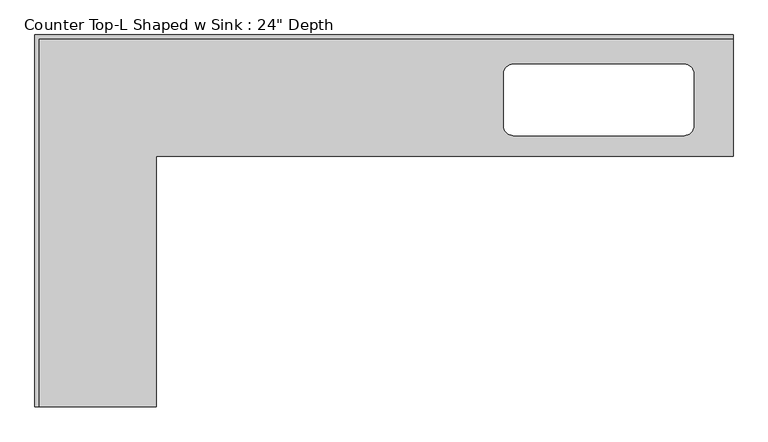
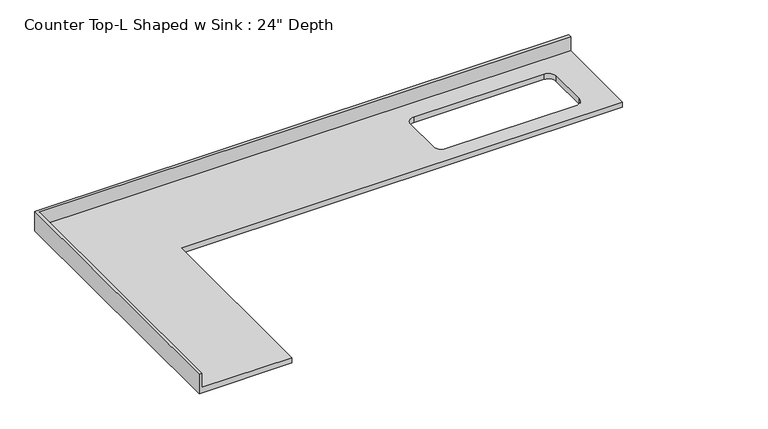
"""IFC4 building model written with IfcOpenShell, lengths in millimetres: furniture geometry."""

from ifc_helpers import new_model, si_unit, frame, origin, place, context, project, spatial, polyline, circle_curve, source, transform, mapped, element, save
from ifc_brep_helpers import plane_surface, revolved_surface, advanced_brep


def furniture_067af109(model_context):
    return source(origin(), model_context, "Body", "AdvancedBrep", [
        advanced_brep(
        [(-565.4622951, -1947.8625, 914.4), (-565.4622951, -635.0, 914.4), (2457.1377049, -635.0, 914.4), (2457.1377049, -19.05, 914.4), (-1181.4122951, -19.05, 914.4), (-1181.4122951, -1947.8625, 914.4), (2200.1132555, -152.693013, 914.4), (2250.9132555, -203.493013, 914.4), (2250.9132555, -477.0306439, 914.4), (2200.1132555, -527.8306439, 914.4), (1306.2231857, -527.8306439, 914.4), (1255.4231857, -477.0306439, 914.4), (1255.4231857, -203.493013, 914.4), (1306.2231857, -152.693013, 914.4), (2457.1377049, 0.0, 876.3), (2457.1377049, -635.0, 876.3), (-565.4622951, -635.0, 876.3), (-565.4622951, -1947.8625, 876.3), (-1200.4622951, -1947.8625, 876.3), (-1200.4622951, 0.0, 876.3), (2200.1132555, -152.693013, 876.3), (1306.2231857, -152.693013, 876.3), (1255.4231857, -203.493013, 876.3), (1255.4231857, -477.0306439, 876.3), (1306.2231857, -527.8306439, 876.3), (2200.1132555, -527.8306439, 876.3), (2250.9132555, -477.0306439, 876.3), (2250.9132555, -203.493013, 876.3), (-1200.4622951, 0.0, 1016.0), (2457.1377049, 0.0, 1016.0), (-1200.4622951, -1947.8625, 1016.0), (-1181.4122951, -1947.8625, 1016.0), (2457.1377049, -19.05, 1016.0), (-1181.4122951, -19.05, 1016.0)],
        [
            (0, 1),
            (1, 2),
            (2, 3),
            (3, 4),
            (4, 5),
            (5, 0),
            (6, 7, circle_curve(frame((2200.1132555, -203.493013, 914.4), z_axis=(0.0, 0.0, -1.0), x_axis=(1.0, 0.0, 0.0)), 50.8)),
            (7, 8),
            (8, 9, circle_curve(frame((2200.1132555, -477.0306439, 914.4), z_axis=(0.0, 0.0, -1.0), x_axis=(1.0, 0.0, 0.0)), 50.8)),
            (9, 10),
            (10, 11, circle_curve(frame((1306.2231857, -477.0306439, 914.4), z_axis=(0.0, 0.0, -1.0), x_axis=(1.0, 0.0, 0.0)), 50.8)),
            (11, 12),
            (12, 13, circle_curve(frame((1306.2231857, -203.493013, 914.4), z_axis=(0.0, 0.0, -1.0), x_axis=(1.0, 0.0, 0.0)), 50.8)),
            (13, 6),
            (14, 15),
            (15, 16),
            (16, 17),
            (17, 18),
            (18, 19),
            (19, 14),
            (20, 21),
            (21, 22, circle_curve(frame((1306.2231857, -203.493013, 876.3), z_axis=(0.0, 0.0, 1.0), x_axis=(1.0, 0.0, 0.0)), 50.8)),
            (22, 23),
            (23, 24, circle_curve(frame((1306.2231857, -477.0306439, 876.3), z_axis=(0.0, 0.0, 1.0), x_axis=(1.0, 0.0, 0.0)), 50.8)),
            (24, 25),
            (25, 26, circle_curve(frame((2200.1132555, -477.0306439, 876.3), z_axis=(0.0, 0.0, 1.0), x_axis=(1.0, 0.0, 0.0)), 50.8)),
            (26, 27),
            (27, 20, circle_curve(frame((2200.1132555, -203.493013, 876.3), z_axis=(0.0, 0.0, 1.0), x_axis=(1.0, 0.0, 0.0)), 50.8)),
            (19, 28),
            (28, 29),
            (29, 14),
            (18, 30),
            (30, 28),
            (17, 0),
            (5, 31),
            (31, 30),
            (16, 1),
            (15, 2),
            (29, 32),
            (32, 3),
            (6, 20),
            (27, 7),
            (26, 8),
            (25, 9),
            (24, 10),
            (23, 11),
            (22, 12),
            (21, 13),
            (31, 33),
            (33, 32),
            (33, 4),
        ],
        [
            plane_surface(frame((-1200.4622951, 0.0, 914.4), z_axis=(0.0, 0.0, 1.0), x_axis=(-1.0, 0.0, 0.0))),
            plane_surface(frame((-1200.4622951, 0.0, 876.3), z_axis=(0.0, 0.0, -1.0), x_axis=(1.0, 0.0, 0.0))),
            plane_surface(frame((2457.1377049, 0.0, 914.4), z_axis=(0.0, 1.0, 0.0), x_axis=(0.0, 0.0, -1.0))),
            plane_surface(frame((-1200.4622951, 0.0, 914.4), z_axis=(-1.0, 0.0, 0.0), x_axis=(0.0, 0.0, -1.0))),
            plane_surface(frame((-1200.4622951, -1947.8625, 914.4), z_axis=(0.0, -1.0, 0.0), x_axis=(0.0, 0.0, -1.0))),
            plane_surface(frame((-565.4622951, -1947.8625, 914.4), z_axis=(1.0, 0.0, 0.0), x_axis=(0.0, 0.0, -1.0))),
            plane_surface(frame((-565.4622951, -635.0, 914.4), z_axis=(0.0, -1.0, 0.0), x_axis=(0.0, 0.0, -1.0))),
            plane_surface(frame((2457.1377049, -635.0, 914.4), z_axis=(1.0, 0.0, 0.0), x_axis=(0.0, 0.0, -1.0))),
            revolved_surface(polyline([(2250.9132555, -203.493013, 876.3), (2250.9132555, -203.493013, 914.4)]), (2200.1132555, -203.493013, 0.0), (0.0, 0.0, -1.0)),
            plane_surface(frame((2250.9132555, -203.493013, 914.4), z_axis=(-1.0, 0.0, 0.0), x_axis=(0.0, 0.0, -1.0))),
            revolved_surface(polyline([(2250.9132555, -477.0306439, 876.3), (2250.9132555, -477.0306439, 914.4)]), (2200.1132555, -477.0306439, 0.0), (0.0, 0.0, -1.0)),
            plane_surface(frame((2200.1132555, -527.8306439, 914.4), z_axis=(0.0, 1.0, 0.0), x_axis=(0.0, 0.0, -1.0))),
            revolved_surface(polyline([(1357.0231856999999, -477.0306439, 876.3), (1357.0231856999999, -477.0306439, 914.4)]), (1306.2231857, -477.0306439, 0.0), (0.0, 0.0, -1.0)),
            plane_surface(frame((1255.4231857, -477.0306439, 914.4), z_axis=(1.0, 0.0, 0.0), x_axis=(0.0, 0.0, -1.0))),
            revolved_surface(polyline([(1357.0231856999999, -203.493013, 876.3), (1357.0231856999999, -203.493013, 914.4)]), (1306.2231857, -203.493013, 0.0), (0.0, 0.0, -1.0)),
            plane_surface(frame((1306.2231857, -152.693013, 914.4), z_axis=(0.0, -1.0, 0.0), x_axis=(0.0, 0.0, -1.0))),
            plane_surface(frame((-1200.4622951, 0.0, 1016.0), z_axis=(0.0, 0.0, 1.0), x_axis=(0.0, -1.0, 0.0))),
            plane_surface(frame((-1200.4622951, -19.05, 1016.0), z_axis=(0.0, -1.0, 0.0), x_axis=(0.0, 0.0, -1.0))),
            plane_surface(frame((-1181.4122951, -1947.8625, 1016.0), z_axis=(1.0, 0.0, 0.0), x_axis=(0.0, 0.0, -1.0))),
        ],
        [
            (0, [[1, 2, 3, 4, 5, 6], [7, 8, 9, 10, 11, 12, 13, 14]]),
            (1, [[15, 16, 17, 18, 19, 20], [21, 22, 23, 24, 25, 26, 27, 28]]),
            (2, [[-20, 29, 30, 31]]),
            (3, [[-19, 32, 33, -29]]),
            (4, [[-32, -18, 34, -6, 35, 36]]),
            (5, [[-1, -34, -17, 37]]),
            (6, [[-2, -37, -16, 38]]),
            (7, [[-15, -31, 39, 40, -3, -38]]),
            (8, [[-7, 41, -28, 42]]),
            (9, [[-8, -42, -27, 43]]),
            (10, [[-9, -43, -26, 44]]),
            (11, [[-10, -44, -25, 45]]),
            (12, [[-11, -45, -24, 46]]),
            (13, [[-12, -46, -23, 47]]),
            (14, [[-13, -47, -22, 48]]),
            (15, [[-14, -48, -21, -41]]),
            (16, [[-33, -36, 49, 50, -39, -30]]),
            (17, [[-40, -50, 51, -4]]),
            (18, [[-49, -35, -5, -51]]),
        ],
    ),
    ])


if __name__ == "__main__":
    model = new_model("IFC4")
    model_context = context("Model", 3, world=origin())
    ifc_project = project(units=[si_unit("LENGTHUNIT", "METRE", prefix="MILLI")], contexts=[model_context])
    site = spatial("IfcSite", under=ifc_project)
    building = spatial("IfcBuilding", under=site)
    placement = place(None, origin())
    furniture_shape = furniture_067af109(model_context)
    element("IfcFurniture", 1, ObjectType="Counter Top-L Shaped w Sink : 24\" Depth", at=placement, inside=building, context=model_context, shape_type="MappedRepresentation", body=[
        mapped(furniture_shape, transform((0.0, 0.0, 0.0), x_axis=(1.0, 0.0, 0.0), y_axis=(0.0, 1.0, 0.0), z_axis=(0.0, 0.0, 1.0))),
    ])
    save(model, "model.ifc")

# Revit data of these elements
# Type "Counter Top-L Shaped w Sink : 24\" Depth"
#   Assembly Code = "C1030400"
#   Counter Thickness = 0' - 1 1/2"
#   Depth = 2' - 1"
#   Height = 3' - 0"
#   Length - Leg 1 [instance default] = 8' - 0"
#   Length - Leg 2 [instance default] = 6' - 0"
#   Sink Location [instance default] = 3' - 0"
#   Sink Location To Wall [instance default] = 0' - 6"
#   Sink Opening Depth [instance default] = 1' - 3"
#   Sink Opening Width [instance default] = 3' - 3"
#   Counter Top Material = none
#   Default Elevation = 0
# Element 1 (IfcFurniture, "Counter Top-L Shaped w Sink : 24\" Depth")
#   Length - Leg 1 = 12' - 0"
#   Length - Leg 2 = 6' - 4 11/16"
#   Sink Location = 8' - 0.6884"
#   Sink Location To Wall = 0' - 6.01154"
#   Sink Opening Depth = 1' - 2.7692"
#   Sink Opening Width = 3' - 3.19252"
#   Materials on its faces: "Counter Top"
# Materials
#   "Counter Top": class "Wood", colour RGB 226 177 128, transparency 0
